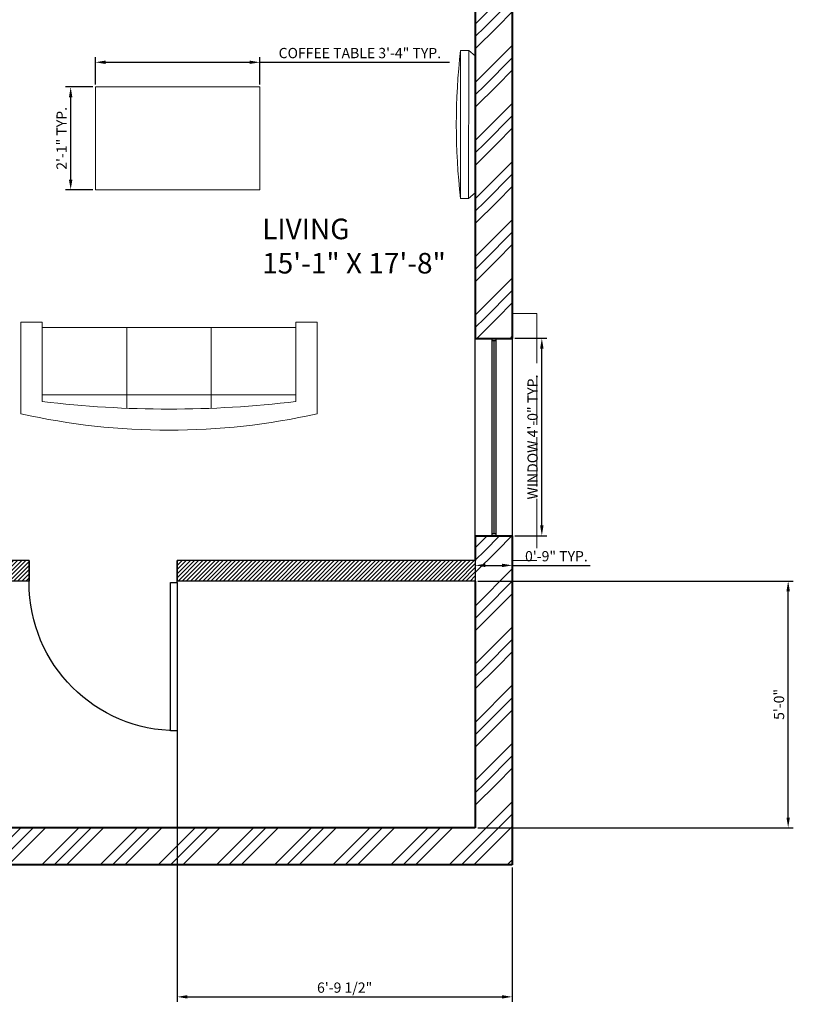
# Model space of a CAD drawing. Units: inches. Extents: x 2443635 to 2446153, y 1826255 to 1827341.
# Tile 9 of 16: x 2444528 to 2444716, y 1826827 to 1827067. Entities that reach past the tile are written whole.
import ezdxf

# ---------------------------------------------------------------- set-up
doc = ezdxf.new("R2010")
doc.units = ezdxf.units.IN
doc.linetypes.add('ACAD_ISO02W100', pattern=[15, 12, -3])
for name, color, linetype, lineweight in [('A-DIMS', 1, 'Continuous', 18), ('A-DOOR', 2, 'Continuous', 25), ('A-EQPM', 8, 'Continuous', 18), ('A-FURN', 6, 'Continuous', 18), ('A-ROOM', 4, 'Continuous', 18), ('A-WALL-EXT', 7, 'Continuous', 40), ('A-WALL-INT', 9, 'Continuous', 30), ('A-WALL-OVHD', 7, 'ACAD_ISO02W100', 18), ('A-WALL-PATT', 8, 'Continuous', 13), ('A-WINDOW', 4, 'Continuous', 25)]:
    doc.layers.add(name, color=color, linetype=linetype, lineweight=lineweight)
doc.styles.get("Standard").update_dxf_attribs({"font": 'arial.ttf'})
doc.dimstyles.new('ISO-25', dxfattribs={"dimtxt": 2.5, "dimasz": 2.5, "dimexe": 1.25, "dimexo": 0.625, "dimtad": 1, "dimlunit": 4, "dimtxsty": 'Standard', "dimcen": 2.5, "dimadec": 0, "dimazin": 0, "dimtfac": 1, "dimtmove": 0, "dimatfit": 3, "dimfxl": 1, "dimarcsym": 0})

# ---------------------------------------------------------------- blocks, each defined once
blk = doc.blocks.new('LCD Monitor Pln')
at = {"layer": 'A-FURN'}
for p, q in [((5656.37, -10564.55), (5660.02, -10561.47)), ((5656.37, -10564.55), (5656.4, -10641.11)), ((5660.02, -10561.47), (5660.05, -10644.19)), ((5664.53, -10561.47), (5660.02, -10561.47)), ((5664.56, -10644.19), (5664.53, -10561.47)), ((5660.05, -10644.19), (5656.4, -10641.11)), ((5660.05, -10644.19), (5664.56, -10644.19))]:
    blk.add_line(p, q, dxfattribs=at)
blk.add_arc((5310.21, -10602.95), 356.75, 353.363, 6.678, dxfattribs=at)
blk = doc.blocks.new('*U3')
for p, q in [((0, 0), (0, -6)), ((-40, 0), (-40, -6))]:
    blk.add_line(p, q)
blk.add_lwpolyline([(0, 0), (0, 40), (-1.75, 40), (-1.75, 0)], close=True)
blk.add_arc((0, 0), 40, 90, 180)
blk = doc.blocks.new('SOFA-3-SEAT')
at = {"transparency": 33554687}
for p, q in [((0, 22.29), (0, 0)), ((72, 0), (72, 22.29)), ((5.14, 0), (5.14, 19.31)), ((25.71, 1.34), (25.71, 20.94)), ((46.29, 1.34), (46.29, 20.94)), ((66.86, 0), (66.86, 19.31)), ((66.86, 17.67), (5.14, 17.67)), ((0, 0), (5.14, 0)), ((66.86, 1.34), (5.14, 1.34)), ((66.86, 0), (72, 0))]:
    blk.add_line(p, q, dxfattribs=at)
for centre, radius, start, end in [((36, -137.71), 164, 77.3196, 102.6804), ((36, -239.71), 260.86, 83.2065, 96.7935)]:
    blk.add_arc(centre, radius, start, end, dxfattribs=at)
blk = doc.blocks.new('COFFEE-TABLE-40X25')
at = {"transparency": 33554687}
for p, q in [((0, 25), (0, 0)), ((40, 25), (0, 25)), ((40, 0), (40, 25)), ((0, 0), (40, 0))]:
    blk.add_line(p, q, dxfattribs=at)
blk = doc.blocks.new('WIN-48-PLAN')
at = {"transparency": 33554687}
for p, q in [((0, 0), (0, 48)), ((0, 48), (9, 48)), ((4, 48), (4, 0)), ((5, 48), (5, 0)), ((9, 48), (9, 0)), ((4, 47.5), (5, 47.5)), ((4.5, 47.5), (4.5, 0.5)), ((5, 0.5), (4, 0.5)), ((9, 0), (0, 0))]:
    blk.add_line(p, q, dxfattribs=at)
blk = doc.blocks.new('WINDOW-HOOD-60-PLAN')
at = {"transparency": 33554687}
for p, q in [((0, 60), (6, 60)), ((6, 60), (6, 0)), ((6, 0), (0, 0))]:
    blk.add_line(p, q, dxfattribs=at)
blk = doc.blocks.new('*D64')
at = {"layer": 'A-DIMS', "color": 0, "lineweight": -2, "transparency": 16777216}
for p, q in [((2444648.18, 1826989.29), (2444656, 1826989.29)), ((2444654.75, 1826943.79), (2444654.75, 1826986.79)), ((2444648.18, 1826941.29), (2444656, 1826941.29))]:
    blk.add_line(p, q, dxfattribs=at)
at = {"layer": 'A-DIMS', "color": 0, "transparency": 16777216}
for points in [[(2444654.34, 1826986.79), (2444655.17, 1826986.79), (2444654.75, 1826989.29)], [(2444654.34, 1826943.79), (2444655.17, 1826943.79), (2444654.75, 1826941.29)]]:
    blk.add_solid(points, dxfattribs=at)
at = {"layer": 'Defpoints', "color": 0, "transparency": 16777216}
for p in [(2444647.55, 1826989.29), (2444654.75, 1826989.29), (2444647.55, 1826941.29)]:
    blk.add_point(p, dxfattribs=at)
at = {"layer": 'A-DIMS', "color": 0, "transparency": 16777216, "insert": (2444652.83, 1826965.29), "char_height": 2.5, "attachment_point": 5, "rotation": 90}
blk.add_mtext('WINDOW 4\'-0" TYP.', dxfattribs=at)
blk = doc.blocks.new('*D65')
at = {"layer": 'A-DIMS', "color": 0, "lineweight": -2, "transparency": 16777216}
for p, q in [((2444638.55, 1826940.66), (2444638.55, 1826932.84)), ((2444647.55, 1826940.66), (2444647.55, 1826932.84)), ((2444641.05, 1826934.09), (2444645.05, 1826934.09)), ((2444647.55, 1826934.09), (2444666.54, 1826934.09))]:
    blk.add_line(p, q, dxfattribs=at)
at = {"layer": 'A-DIMS', "color": 0, "transparency": 16777216}
for points in [[(2444641.05, 1826934.5), (2444641.05, 1826933.67), (2444638.55, 1826934.09)], [(2444645.05, 1826934.5), (2444645.05, 1826933.67), (2444647.55, 1826934.09)]]:
    blk.add_solid(points, dxfattribs=at)
at = {"layer": 'Defpoints', "color": 0, "transparency": 16777216}
for p in [(2444638.55, 1826941.29), (2444647.55, 1826941.29), (2444647.55, 1826934.09)]:
    blk.add_point(p, dxfattribs=at)
at = {"layer": 'A-DIMS', "color": 0, "transparency": 16777216, "insert": (2444658.3, 1826935.99), "char_height": 2.5, "attachment_point": 5}
blk.add_mtext('0\'-9" TYP.', dxfattribs=at)
blk = doc.blocks.new('*D72')
at = {"layer": 'A-DIMS', "color": 0, "lineweight": -2, "transparency": 16777216}
for p, q in [((2444546.18, 1827051.03), (2444546.18, 1827057.65)), ((2444586.18, 1827051.03), (2444586.18, 1827057.65)), ((2444548.68, 1827056.4), (2444583.68, 1827056.4)), ((2444586.18, 1827056.4), (2444632.31, 1827056.4))]:
    blk.add_line(p, q, dxfattribs=at)
at = {"layer": 'A-DIMS', "color": 0, "transparency": 16777216}
for points in [[(2444548.68, 1827056.82), (2444548.68, 1827055.99), (2444546.18, 1827056.4)], [(2444583.68, 1827056.82), (2444583.68, 1827055.99), (2444586.18, 1827056.4)]]:
    blk.add_solid(points, dxfattribs=at)
at = {"layer": 'Defpoints', "color": 0, "transparency": 16777216}
for p in [(2444586.18, 1827056.4), (2444546.18, 1827050.4), (2444586.18, 1827050.4)]:
    blk.add_point(p, dxfattribs=at)
at = {"layer": 'A-DIMS', "color": 0, "transparency": 16777216, "insert": (2444610.5, 1827058.32), "char_height": 2.5, "attachment_point": 5}
blk.add_mtext('COFFEE TABLE 3\'-4" TYP.', dxfattribs=at)
blk = doc.blocks.new('*D73')
at = {"layer": 'A-DIMS', "color": 0, "lineweight": -2, "transparency": 16777216}
for p, q in [((2444545.56, 1827050.4), (2444538.93, 1827050.4)), ((2444540.18, 1827027.9), (2444540.18, 1827047.9)), ((2444545.56, 1827025.4), (2444538.93, 1827025.4))]:
    blk.add_line(p, q, dxfattribs=at)
at = {"layer": 'A-DIMS', "color": 0, "transparency": 16777216}
for points in [[(2444539.76, 1827047.9), (2444540.6, 1827047.9), (2444540.18, 1827050.4)], [(2444539.76, 1827027.9), (2444540.6, 1827027.9), (2444540.18, 1827025.4)]]:
    blk.add_solid(points, dxfattribs=at)
at = {"layer": 'Defpoints', "color": 0, "transparency": 16777216}
for p in [(2444540.18, 1827050.4), (2444546.18, 1827050.4), (2444546.18, 1827025.4)]:
    blk.add_point(p, dxfattribs=at)
at = {"layer": 'A-DIMS', "color": 0, "transparency": 16777216, "insert": (2444538.3, 1827037.9), "char_height": 2.5, "attachment_point": 5, "rotation": 90}
blk.add_mtext('2\'-1" TYP.', dxfattribs=at)
blk = doc.blocks.new('*D97')
at = {"layer": 'A-DIMS', "color": 0, "lineweight": -2, "transparency": 16777216}
for p, q in [((2444639.18, 1826930.29), (2444715.9, 1826930.29)), ((2444714.65, 1826872.79), (2444714.65, 1826927.79)), ((2444639.18, 1826870.29), (2444715.9, 1826870.29))]:
    blk.add_line(p, q, dxfattribs=at)
at = {"layer": 'A-DIMS', "color": 0, "transparency": 16777216}
for points in [[(2444714.24, 1826927.79), (2444715.07, 1826927.79), (2444714.65, 1826930.29)], [(2444714.24, 1826872.79), (2444715.07, 1826872.79), (2444714.65, 1826870.29)]]:
    blk.add_solid(points, dxfattribs=at)
at = {"layer": 'Defpoints', "color": 0, "transparency": 16777216}
for p in [(2444638.55, 1826930.29), (2444714.65, 1826930.29), (2444638.55, 1826870.29)]:
    blk.add_point(p, dxfattribs=at)
at = {"layer": 'A-DIMS', "color": 0, "transparency": 16777216, "insert": (2444712.75, 1826900.29), "char_height": 2.5, "attachment_point": 5, "rotation": 90}
blk.add_mtext('5\'-0"', dxfattribs=at)
blk = doc.blocks.new('*D98')
at = {"layer": 'A-DIMS', "color": 0, "lineweight": -2, "transparency": 16777216}
for p, q in [((2444566.05, 1826929.66), (2444566.05, 1826827.94)), ((2444647.55, 1826860.66), (2444647.55, 1826827.94)), ((2444568.55, 1826829.19), (2444645.05, 1826829.19))]:
    blk.add_line(p, q, dxfattribs=at)
at = {"layer": 'A-DIMS', "color": 0, "transparency": 16777216}
for points in [[(2444568.55, 1826829.6), (2444568.55, 1826828.77), (2444566.05, 1826829.19)], [(2444645.05, 1826829.6), (2444645.05, 1826828.77), (2444647.55, 1826829.19)]]:
    blk.add_solid(points, dxfattribs=at)
at = {"layer": 'Defpoints', "color": 0, "transparency": 16777216}
for p in [(2444566.05, 1826930.29), (2444647.55, 1826861.29), (2444647.55, 1826829.19)]:
    blk.add_point(p, dxfattribs=at)
at = {"layer": 'A-DIMS', "color": 0, "transparency": 16777216, "insert": (2444606.8, 1826831.11), "char_height": 2.5, "attachment_point": 5}
blk.add_mtext('6\'-9 1/2"', dxfattribs=at)

msp = doc.modelspace()

# ---------------------------------------------------------------- hatches: boundary and pattern name
at = {"layer": 'A-WALL-PATT'}
h = msp.add_hatch(dxfattribs=at)
h.set_pattern_fill('GOST_GROUND', color=256)
h.paths.add_polyline_path([(2444332.553, 1827147.288), (2444332.553, 1827152.288), (2444332.553, 1827161.288), (2444328.953, 1827161.288), (2444323.553, 1827161.288), (2444323.553, 1826984.288), (2444332.553, 1826984.288), (2444332.553, 1827062.288), (2444332.553, 1827067.288)])
h.paths.add_polyline_path([(2444332.553, 1826948.288), (2444323.553, 1826948.288), (2444323.553, 1826861.288), (2444374.553, 1826861.288), (2444374.553, 1826870.288), (2444332.553, 1826870.288)])
h.paths.add_polyline_path([(2444647.553, 1826941.288), (2444638.553, 1826941.288), (2444638.553, 1826935.288), (2444638.553, 1826930.288), (2444638.553, 1826870.288), (2444457.553, 1826870.288), (2444452.553, 1826870.288), (2444410.553, 1826870.288), (2444410.553, 1826861.288), (2444647.553, 1826861.288)])
h.paths.add_polyline_path([(2444647.553, 1827161.288), (2444638.553, 1827161.288), (2444638.553, 1827152.288), (2444638.553, 1827147.288), (2444638.553, 1826989.288), (2444647.553, 1826989.288)])
h.paths.add_polyline_path([(2444647.553, 1827305.288), (2444494.553, 1827305.288), (2444494.553, 1827296.288), (2444498.051, 1827296.288), (2444638.553, 1827296.288), (2444638.553, 1827254.288), (2444647.553, 1827254.288)])
h.paths.add_polyline_path([(2444476.553, 1827305.288), (2444323.553, 1827305.288), (2444323.553, 1827254.288), (2444332.553, 1827254.288), (2444332.553, 1827296.288), (2444346.141, 1827296.288), (2444476.553, 1827296.288)])
h.paths.add_polyline_path([(2444323.553, 1827305.288), (2444282.553, 1827305.288), (2444282.553, 1827147.459), (2444323.553, 1827147.459), (2444323.553, 1827152.459), (2444287.553, 1827152.459), (2444287.553, 1827300.288), (2444323.553, 1827300.288)])
h.paths.add_polyline_path([(2444688.553, 1827305.288), (2444647.553, 1827305.288), (2444647.553, 1827300.288), (2444683.553, 1827300.288), (2444683.553, 1827152.362), (2444647.553, 1827152.362), (2444647.553, 1827147.362), (2444688.553, 1827147.362)])
h = msp.add_hatch(dxfattribs=at)
h.set_pattern_fill('JIS_WOOD', color=256)
h.paths.add_polyline_path([(2444481.553, 1827095.288), (2444476.553, 1827095.288), (2444476.553, 1827067.288), (2444332.553, 1827067.288), (2444332.553, 1827062.288), (2444481.553, 1827062.288)])
h.paths.add_polyline_path([(2444457.553, 1827020.288), (2444452.553, 1827020.288), (2444452.553, 1826870.288), (2444457.553, 1826870.288), (2444457.553, 1826930.288), (2444530.053, 1826930.288), (2444530.053, 1826935.288), (2444457.553, 1826935.288)])
h.paths.add_polyline_path([(2444457.553, 1827062.288), (2444452.553, 1827062.288), (2444452.553, 1827056.288), (2444457.553, 1827056.288)])
h.paths.add_polyline_path([(2444638.553, 1826935.288), (2444566.053, 1826935.288), (2444566.053, 1826930.288), (2444638.553, 1826930.288)])
h.paths.add_polyline_path([(2444638.553, 1827152.288), (2444518.553, 1827152.288), (2444518.553, 1827156.288), (2444513.553, 1827156.288), (2444513.553, 1827147.288), (2444638.553, 1827147.288)])
h.paths.add_polyline_path([(2444518.553, 1827296.288), (2444513.553, 1827296.288), (2444513.553, 1827224.288), (2444507.553, 1827224.288), (2444507.553, 1827223.788), (2444507.553, 1827219.288), (2444513.553, 1827219.288), (2444513.553, 1827192.288), (2444518.553, 1827192.288)])
h.paths.add_polyline_path([(2444477.553, 1827223.788, -0.0041669), (2444477.557, 1827224.288), (2444457.553, 1827224.288), (2444457.553, 1827296.288), (2444452.553, 1827296.288), (2444452.553, 1827192.288), (2444457.553, 1827192.288), (2444457.553, 1827219.288), (2444477.553, 1827219.288)])
h.paths.add_polyline_path([(2444481.553, 1827152.288), (2444332.553, 1827152.288), (2444332.553, 1827147.288), (2444476.553, 1827147.288), (2444476.553, 1827137.288), (2444481.553, 1827137.288)])

# ---------------------------------------------------------------- linework, layer by layer
at = {"layer": 'A-WALL-EXT'}
for p, q in [((2444647.553, 1827162.338), (2444647.553, 1826989.288)), ((2444638.553, 1827147.288), (2444638.553, 1826989.288)), ((2444638.553, 1826989.288), (2444647.553, 1826989.288)), ((2444638.553, 1826941.288), (2444647.553, 1826941.288)), ((2444638.553, 1826941.288), (2444638.553, 1826935.288)), ((2444647.553, 1826941.288), (2444647.553, 1826861.288)), ((2444638.553, 1826930.288), (2444638.553, 1826870.288)), ((2444638.553, 1826870.288), (2444457.553, 1826870.288)), ((2444647.553, 1826861.288), (2444410.553, 1826861.288))]:
    msp.add_line(p, q, dxfattribs=at)
at = {"layer": 'A-WALL-INT'}
for p, q in [((2444530.053, 1826935.288), (2444457.553, 1826935.288)), ((2444530.053, 1826935.288), (2444530.053, 1826930.288)), ((2444638.553, 1826935.288), (2444566.053, 1826935.288)), ((2444566.053, 1826935.288), (2444566.053, 1826930.288)), ((2444638.553, 1826935.288), (2444638.553, 1826930.288)), ((2444530.053, 1826930.288), (2444457.553, 1826930.288)), ((2444638.553, 1826930.288), (2444566.053, 1826930.288))]:
    msp.add_line(p, q, dxfattribs=at)
at = {"layer": 'A-WINDOW'}
for p, q in [((2444638.553, 1826989.288), (2444647.553, 1826989.288)), ((2444647.553, 1826941.288), (2444638.553, 1826941.288))]:
    msp.add_line(p, q, dxfattribs=at)

# ---------------------------------------------------------------- block references
at = {"layer": 'A-DOOR', "xscale": -0.9, "yscale": 0.9, "zscale": 0.9, "rotation": 180}
msp.add_blockref('*U3', (2444566.053, 1826929.888), dxfattribs=at)
at = {"layer": 'A-EQPM', "xscale": -0.4352145044351718, "yscale": 0.4352145044351718, "zscale": 0.4352145044351718}
msp.add_blockref('LCD Monitor Pln', (2447100.293, 1831655.793), dxfattribs=at)
at = {"layer": 'A-FURN', "transparency": 33554687}
msp.add_blockref('COFFEE-TABLE-40X25', (2444546.181, 1827025.403), dxfattribs=at)
at = {"layer": 'A-FURN', "transparency": 33554687, "rotation": 180.0000246857248}
msp.add_blockref('SOFA-3-SEAT', (2444600.094, 1826993.237), dxfattribs=at)
at = {"layer": 'A-WALL-OVHD', "transparency": 33554687}
msp.add_blockref('WINDOW-HOOD-60-PLAN', (2444647.553, 1826935.288), dxfattribs=at)
at = {"layer": 'A-WINDOW', "transparency": 33554687}
msp.add_blockref('WIN-48-PLAN', (2444638.553, 1826941.288), dxfattribs=at)

# ---------------------------------------------------------------- texts
at = {"layer": 'A-ROOM', "insert": (2444586.736, 1827018.388), "char_height": 5, "attachment_point": 1}
msp.add_mtext_dynamic_manual_height_columns('LIVING\\P15\'-1" X 17\'-8"', width=52.37406, gutter_width=12.5, heights=[0], dxfattribs=at)

# ---------------------------------------------------------------- dimensions: what is measured, and where the dimension line sits
at = {"layer": 'A-DIMS', "transparency": 33554687}
for base, p1, p2, text, picture, middle in [((2444586.182, 1827056.403), (2444546.182, 1827050.403), (2444586.182, 1827050.403), 'COFFEE TABLE <> TYP.', '*D72', (2444610.496, 1827058.322)), ((2444647.553, 1826934.088), (2444638.553, 1826941.288), (2444647.553, 1826941.288), '<> TYP.', '*D65', (2444658.297, 1826935.989))]:
    dim = msp.add_linear_dim(base=base, p1=p1, p2=p2, text=text, dimstyle='ISO-25', override={"dimdec": 1, "dimlfac": 1, "dimrnd": 0, "dimzin": 1, "dimdsep": 46, "dimlunit": 4, "dimfrac": 2}, dxfattribs=at)
    dim.commit()
    dim.dimension.update_dxf_attribs({"geometry": picture, "text_midpoint": middle})
for base, p1, p2, text, picture, middle in [((2444540.182, 1827050.403), (2444546.182, 1827025.403), (2444546.182, 1827050.403), '<> TYP.', '*D73', (2444538.301, 1827037.903)), ((2444654.753, 1826989.288), (2444647.553, 1826941.288), (2444647.553, 1826989.288), 'WINDOW <> TYP.', '*D64', (2444652.834, 1826965.288))]:
    dim = msp.add_linear_dim(base=base, p1=p1, p2=p2, angle=90, text=text, dimstyle='ISO-25', override={"dimdec": 1, "dimlfac": 1, "dimrnd": 0, "dimzin": 1, "dimdsep": 46, "dimlunit": 4, "dimfrac": 2}, dxfattribs=at)
    dim.commit()
    dim.dimension.update_dxf_attribs({"geometry": picture, "text_midpoint": middle})
dim = msp.add_linear_dim(base=(2444647.553, 1826829.188), p1=(2444566.053, 1826930.288), p2=(2444647.553, 1826861.288), dimstyle='ISO-25', override={"dimdec": 1, "dimlfac": 1, "dimrnd": 0, "dimzin": 1, "dimdsep": 46, "dimlunit": 4, "dimfrac": 2}, dxfattribs=at)
dim.commit()
dim.dimension.update_dxf_attribs({"geometry": '*D98', "text_midpoint": (2444606.803, 1826831.106)})
dim = msp.add_linear_dim(base=(2444714.653, 1826930.288), p1=(2444638.553, 1826870.288), p2=(2444638.553, 1826930.288), angle=90, dimstyle='ISO-25', override={"dimdec": 1, "dimlfac": 1, "dimrnd": 0, "dimzin": 1, "dimdsep": 46, "dimlunit": 4, "dimfrac": 2}, dxfattribs=at)
dim.commit()
dim.dimension.update_dxf_attribs({"geometry": '*D97', "text_midpoint": (2444712.751, 1826900.288)})

doc.saveas('drawing.dxf')
